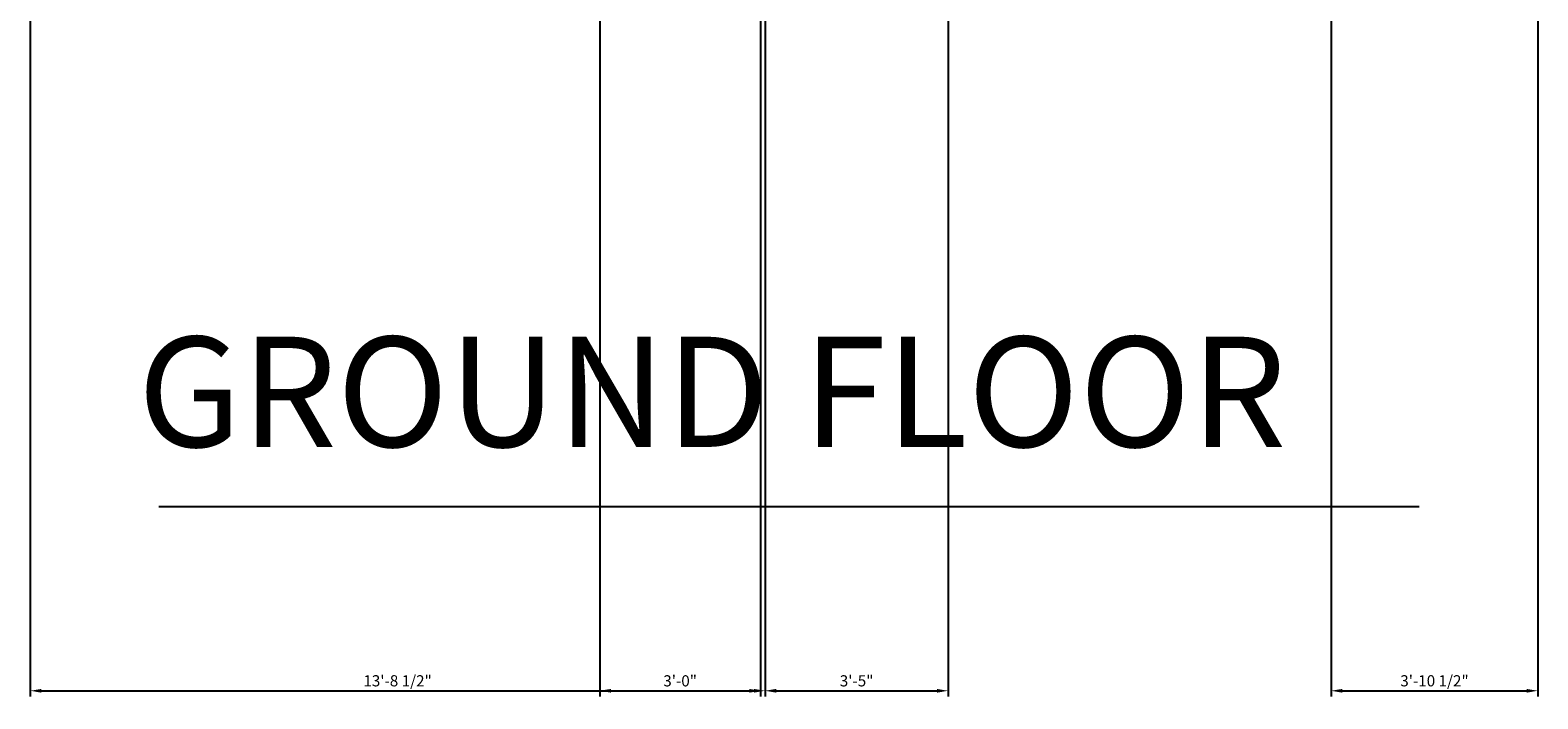
# Model space of a CAD drawing. Units: inches. Extents: x 2691 to 8091, y 3734 to 9067.
# Tile 1 of 5: x 2742 to 3079, y 3734 to 3884. Entities that reach past the tile are written whole.
import ezdxf

# ---------------------------------------------------------------- set-up
doc = ezdxf.new("R2010")
doc.units = ezdxf.units.IN
doc.layers.add('A-ANNO-DIMS', color=2, linetype='Continuous', lineweight=18)
doc.layers.add('A-ANNO-TEXT', color=7, linetype='Continuous', lineweight=25)
doc.styles.get("Standard").update_dxf_attribs({"font": 'arial.ttf'})
doc.dimstyles.new('ISO-25', dxfattribs={"dimtxt": 2.5, "dimasz": 2.5, "dimexe": 1.25, "dimexo": 0.625, "dimtad": 1, "dimdec": 1, "dimlunit": 3, "dimtxsty": 'Standard', "dimcen": 2.5, "dimadec": 0, "dimazin": 0, "dimtfac": 1, "dimtdec": 1, "dimtmove": 0, "dimatfit": 3, "dimfxl": 1, "dimarcsym": 0})

# ---------------------------------------------------------------- blocks, each defined once
blk = doc.blocks.new('*D56')
at = {"layer": 'A-ANNO-DIMS', "color": 0, "lineweight": -2, "transparency": 16777216}
for p, q in [((2741.96, 4003.19), (2741.96, 3735.06)), ((2906.46, 4003.19), (2906.46, 3735.06)), ((2744.46, 3736.31), (2903.96, 3736.31))]:
    blk.add_line(p, q, dxfattribs=at)
at = {"layer": 'A-ANNO-DIMS', "color": 0, "transparency": 16777216}
for points in [[(2744.46, 3736.72), (2744.46, 3735.89), (2741.96, 3736.31)], [(2903.96, 3736.72), (2903.96, 3735.89), (2906.46, 3736.31)]]:
    blk.add_solid(points, dxfattribs=at)
at = {"layer": 'Defpoints', "color": 0, "transparency": 16777216}
for p in [(2741.96, 4003.82), (2906.46, 4003.82), (2906.46, 3736.31)]:
    blk.add_point(p, dxfattribs=at)
at = {"layer": 'A-ANNO-DIMS', "color": 0, "transparency": 16777216, "insert": (2824.21, 3738.22), "char_height": 2.5, "attachment_point": 5}
blk.add_mtext('13\'-8 1/2"', dxfattribs=at)
blk = doc.blocks.new('*D57')
at = {"layer": 'A-ANNO-DIMS', "color": 0, "lineweight": -2, "transparency": 16777216}
for p, q in [((2906.46, 4003.19), (2906.46, 3735.06)), ((2947.46, 4003.19), (2947.46, 3735.06)), ((2908.96, 3736.31), (2944.96, 3736.31))]:
    blk.add_line(p, q, dxfattribs=at)
at = {"layer": 'A-ANNO-DIMS', "color": 0, "transparency": 16777216}
for points in [[(2908.96, 3736.72), (2908.96, 3735.89), (2906.46, 3736.31)], [(2944.96, 3736.72), (2944.96, 3735.89), (2947.46, 3736.31)]]:
    blk.add_solid(points, dxfattribs=at)
at = {"layer": 'Defpoints', "color": 0, "transparency": 16777216}
for p in [(2906.46, 4003.82), (2947.46, 4003.82), (2947.46, 3736.31)]:
    blk.add_point(p, dxfattribs=at)
at = {"layer": 'A-ANNO-DIMS', "color": 0, "transparency": 16777216, "insert": (2926.96, 3738.21), "char_height": 2.5, "attachment_point": 5}
blk.add_mtext('3\'-5"', dxfattribs=at)
blk = doc.blocks.new('*D58')
at = {"layer": 'A-ANNO-DIMS', "color": 0, "lineweight": -2, "transparency": 16777216}
for p, q in [((3033.17, 4003.19), (3033.17, 3735.06)), ((3079.46, 4003.19), (3079.46, 3735.06)), ((3035.67, 3736.31), (3076.96, 3736.31))]:
    blk.add_line(p, q, dxfattribs=at)
at = {"layer": 'A-ANNO-DIMS', "color": 0, "transparency": 16777216}
for points in [[(3035.67, 3736.72), (3035.67, 3735.89), (3033.17, 3736.31)], [(3076.96, 3736.72), (3076.96, 3735.89), (3079.46, 3736.31)]]:
    blk.add_solid(points, dxfattribs=at)
at = {"layer": 'Defpoints', "color": 0, "transparency": 16777216}
for p in [(3033.17, 4003.82), (3079.46, 4003.82), (3079.46, 3736.31)]:
    blk.add_point(p, dxfattribs=at)
at = {"layer": 'A-ANNO-DIMS', "color": 0, "transparency": 16777216, "insert": (3056.32, 3738.22), "char_height": 2.5, "attachment_point": 5}
blk.add_mtext('3\'-10 1/2"', dxfattribs=at)
blk = doc.blocks.new('*D59')
at = {"layer": 'A-ANNO-DIMS', "color": 0, "lineweight": -2, "transparency": 16777216}
for p, q in [((2869.46, 4415.69), (2869.46, 3735.06)), ((2905.46, 4415.69), (2905.46, 3735.06)), ((2871.96, 3736.31), (2902.96, 3736.31))]:
    blk.add_line(p, q, dxfattribs=at)
at = {"layer": 'A-ANNO-DIMS', "color": 0, "transparency": 16777216}
for points in [[(2871.96, 3736.72), (2871.96, 3735.89), (2869.46, 3736.31)], [(2902.96, 3736.72), (2902.96, 3735.89), (2905.46, 3736.31)]]:
    blk.add_solid(points, dxfattribs=at)
at = {"layer": 'Defpoints', "color": 0, "transparency": 16777216}
for p in [(2869.46, 4416.32), (2905.46, 4416.32), (2905.46, 3736.31)]:
    blk.add_point(p, dxfattribs=at)
at = {"layer": 'A-ANNO-DIMS', "color": 0, "transparency": 16777216, "insert": (2887.46, 3738.21), "char_height": 2.5, "attachment_point": 5}
blk.add_mtext('3\'-0"', dxfattribs=at)

msp = doc.modelspace()

# ---------------------------------------------------------------- linework, layer by layer
at = {"layer": 'A-ANNO-TEXT'}
msp.add_line((2770.8, 3777.56), (3052.88, 3777.56), dxfattribs=at)

# ---------------------------------------------------------------- texts
msp.add_text('GROUND FLOOR', height=24.6832, dxfattribs=at).set_placement((2766.04, 3790.93))

# ---------------------------------------------------------------- dimensions: what is measured, and where the dimension line sits
at = {"layer": 'A-ANNO-DIMS'}
for base, p1, p2, picture, middle in [((2905.46, 3736.31), (2869.46, 4416.32), (2905.46, 4416.32), '*D59', (2887.46, 3738.21)), ((2906.46, 3736.31), (2741.96, 4003.82), (2906.46, 4003.82), '*D56', (2824.21, 3738.22)), ((2947.46, 3736.31), (2906.46, 4003.82), (2947.46, 4003.82), '*D57', (2926.96, 3738.21)), ((3079.46, 3736.31), (3033.17, 4003.82), (3079.46, 4003.82), '*D58', (3056.32, 3738.22))]:
    dim = msp.add_linear_dim(base=base, p1=p1, p2=p2, dimstyle='ISO-25', override={"dimdec": 1, "dimlfac": 1, "dimrnd": 0, "dimzin": 1, "dimdsep": 46, "dimlunit": 4, "dimfrac": 2}, dxfattribs=at)
    dim.commit()
    dim.dimension.update_dxf_attribs({"geometry": picture, "text_midpoint": middle})

doc.saveas('drawing.dxf')
